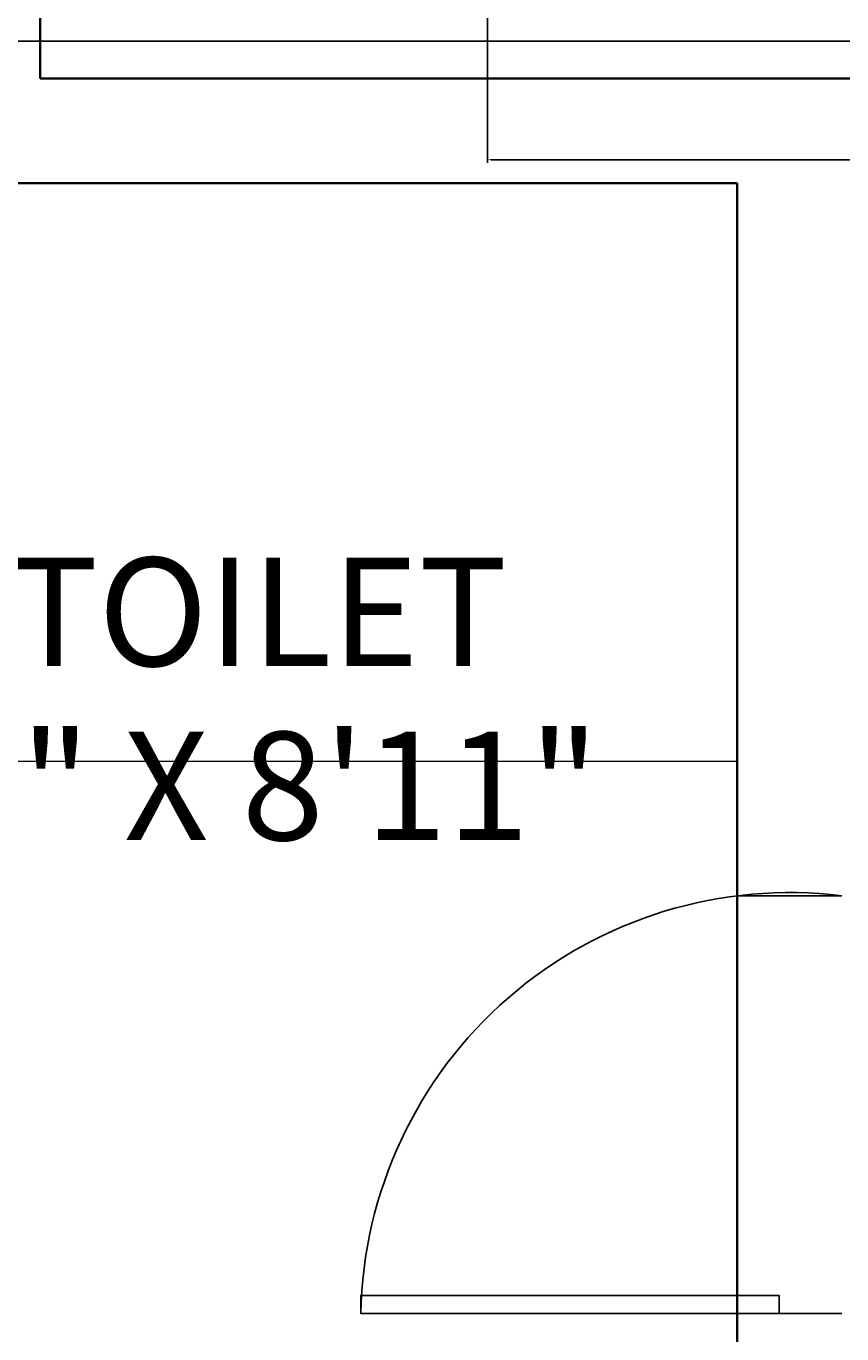
# Model space of a CAD drawing. Units: inches. Extents: x -61 to 1599, y -1316 to 257.
# Tile 62 of 204: x 119 to 166, y -241 to -166. Entities that reach past the tile are written whole.
import ezdxf

# ---------------------------------------------------------------- set-up
doc = ezdxf.new("R2010")
doc.units = ezdxf.units.IN
doc.header["$MEASUREMENT"] = 0
doc.linetypes.add('ACAD_ISO02W100', pattern=[15, 12, -3])
for name, color, linetype, lineweight in [('A-ANNO-DIMS', 2, 'Continuous', 18), ('A-AREA-IDEN', 1, 'Continuous', 18), ('A-FLOR-FIXT', 8, 'Continuous', 18), ('A-WALL-JAMB', 4, 'ACAD_ISO02W100', 25), ('DOORS', 2, 'Continuous', 25), ('WALLS', 4, 'Continuous', 35)]:
    doc.layers.add(name, color=color, linetype=linetype, lineweight=lineweight)
doc.styles.get("Standard").update_dxf_attribs({"font": 'arial.ttf'})
doc.dimstyles.get("Standard").update_dxf_attribs({"dimtxt": 0.18, "dimasz": 0.18, "dimexe": 0.18, "dimexo": 0.0625, "dimgap": 0.09, "dimtad": 0, "dimtih": 1, "dimtoh": 1, "dimdec": 0, "dimzin": 0, "dimdsep": 46, "dimlunit": 3, "dimtxsty": 'Standard', "dimcen": 0.09, "dimadec": 0, "dimazin": 0, "dimtfac": 1, "dimtdec": 0, "dimtofl": 0, "dimtmove": 0, "dimatfit": 3, "dimfxl": 1, "dimtolj": 1, "dimtzin": 0, "dimarcsym": 0})

# ---------------------------------------------------------------- blocks, each defined once
blk = doc.blocks.new('DOOR-SWING-24')
blk.add_line((0, 0), (0, 3.6))
blk.add_lwpolyline([(0, 0), (0, -24), (1.05, -24), (1.05, 0)], close=True)
blk.add_arc((-0.441, 0.618), 24.622, 271.02591, 6.95592)
blk = doc.blocks.new('*D670')
at = {"layer": 'A-ANNO-DIMS', "color": 0, "lineweight": -2, "transparency": 16777216}
for p, q in [((145.375, -161.442), (145.375, -174.159)), ((229.375, -161.442), (229.375, -174.159)), ((145.555, -173.979), (186.47, -173.979)), ((229.195, -173.979), (188.279, -173.979))]:
    blk.add_line(p, q, dxfattribs=at)
at = {"layer": 'A-ANNO-DIMS', "color": 0, "transparency": 16777216}
for points in [[(145.555, -173.949), (145.555, -174.009), (145.375, -173.979)], [(229.195, -173.949), (229.195, -174.009), (229.375, -173.979)]]:
    blk.add_solid(points, dxfattribs=at)
at = {"layer": 'DEFPOINTS', "color": 0, "transparency": 16777216}
for p in [(145.375, -161.379), (229.375, -161.379), (229.375, -173.979)]:
    blk.add_point(p, dxfattribs=at)
at = {"layer": 'A-ANNO-DIMS', "color": 0, "transparency": 16777216, "insert": (187.375, -173.979), "char_height": 0.18, "attachment_point": 5}
blk.add_mtext('\\A1;SOFA 84 TYP.', dxfattribs=at)
blk = doc.blocks.new('*D687')
at = {"layer": 'A-ANNO-DIMS', "color": 0, "lineweight": -2, "transparency": 16777216}
for p, q in [((289.418, 181.677), (-61.077, 181.677)), ((-60.897, 181.497), (-60.897, -528.952)), ((-60.897, -1239.765), (-60.897, -529.316)), ((319.64, -1239.945), (-61.077, -1239.945))]:
    blk.add_line(p, q, dxfattribs=at)
at = {"layer": 'A-ANNO-DIMS', "color": 0, "transparency": 16777216}
for points in [[(-60.927, 181.497), (-60.867, 181.497), (-60.897, 181.677)], [(-60.927, -1239.765), (-60.867, -1239.765), (-60.897, -1239.945)]]:
    blk.add_solid(points, dxfattribs=at)
at = {"layer": 'DEFPOINTS', "color": 0, "transparency": 16777216}
for p in [(289.481, 181.677), (-60.897, -1239.945), (319.703, -1239.945)]:
    blk.add_point(p, dxfattribs=at)
at = {"layer": 'A-ANNO-DIMS', "color": 0, "transparency": 16777216, "insert": (-60.897, -529.134), "char_height": 0.18, "attachment_point": 5}
blk.add_mtext('\\A1;1421.6', dxfattribs=at)
blk = doc.blocks.new('*D699')
at = {"layer": 'A-ANNO-DIMS', "color": 0, "lineweight": -2, "transparency": 16777216}
for p, q in [((835.64, -167.169), (-61.077, -167.169)), ((-60.897, -167.349), (-60.897, -306.726)), ((-60.897, -446.466), (-60.897, -307.09)), ((841.64, -446.646), (-61.077, -446.646))]:
    blk.add_line(p, q, dxfattribs=at)
at = {"layer": 'A-ANNO-DIMS', "color": 0, "transparency": 16777216}
for points in [[(-60.927, -167.349), (-60.867, -167.349), (-60.897, -167.169)], [(-60.927, -446.466), (-60.867, -446.466), (-60.897, -446.646)]]:
    blk.add_solid(points, dxfattribs=at)
at = {"layer": 'DEFPOINTS', "color": 0, "transparency": 16777216}
for p in [(835.703, -167.169), (-60.897, -446.646), (841.703, -446.646)]:
    blk.add_point(p, dxfattribs=at)
at = {"layer": 'A-ANNO-DIMS', "color": 0, "transparency": 16777216, "insert": (-60.897, -306.908), "char_height": 0.18, "attachment_point": 5}
blk.add_mtext('\\A1;279.5', dxfattribs=at)
blk = doc.blocks.new('*D700')
at = {"layer": 'A-ANNO-DIMS', "color": 0, "lineweight": -2, "transparency": 16777216}
for p, q in [((14.703, -616.882), (14.703, 257.457)), ((14.883, 257.277), (96.772, 257.277)), ((179.572, 257.277), (97.683, 257.277)), ((179.752, -616.882), (179.752, 257.457))]:
    blk.add_line(p, q, dxfattribs=at)
at = {"layer": 'A-ANNO-DIMS', "color": 0, "transparency": 16777216}
for points in [[(14.883, 257.307), (14.883, 257.247), (14.703, 257.277)], [(179.572, 257.307), (179.572, 257.247), (179.752, 257.277)]]:
    blk.add_solid(points, dxfattribs=at)
at = {"layer": 'DEFPOINTS', "color": 0, "transparency": 16777216}
for p in [(179.752, 257.277), (14.703, -616.945), (179.752, -616.945)]:
    blk.add_point(p, dxfattribs=at)
at = {"layer": 'A-ANNO-DIMS', "color": 0, "transparency": 16777216, "insert": (97.227, 257.277), "char_height": 0.18, "attachment_point": 5}
blk.add_mtext('\\A1;165.05', dxfattribs=at)

msp = doc.modelspace()

# ---------------------------------------------------------------- linework, layer by layer
at = {"layer": 'A-FLOR-FIXT'}
msp.add_line((87.7028, -208.5091), (159.7028, -208.5091), dxfattribs=at)
at = {"layer": 'A-WALL-JAMB'}
for p, q in [((165.7028, -216.2369), (159.7028, -216.2369)), ((165.7028, -240.2369), (159.7028, -240.2369))]:
    msp.add_line(p, q, dxfattribs=at)
at = {"layer": 'WALLS'}
for p, q in [((119.7028, -169.3229), (119.7028, -13.3229)), ((119.7028, -169.3229), (234.7028, -169.3229)), ((87.7028, -175.3229), (159.7028, -175.3229)), ((159.7028, -282.3229), (159.7028, -175.3229))]:
    msp.add_line(p, q, dxfattribs=at)

# ---------------------------------------------------------------- block references
at = {"layer": 'DOORS', "extrusion": (0, 0, -1), "zscale": -1, "rotation": 89.99999999999957}
msp.add_blockref('DOOR-SWING-24', (-162.1028, -240.2369), dxfattribs=at)

# ---------------------------------------------------------------- texts
at = {"layer": 'A-AREA-IDEN'}
for s, p in [(' M . TOILET', (102.978, -203.0507)), ('  6\'0" X 8\'11"', (102.978, -213.0484))]:
    msp.add_text(s, height=6.223643, dxfattribs=at).set_placement(p)

# ---------------------------------------------------------------- dimensions: what is measured, and where the dimension line sits
at = {"layer": 'A-ANNO-DIMS'}
dim = msp.add_linear_dim(base=(179.7521, 257.2771), p1=(14.7028, -616.9446), p2=(179.7521, -616.9446), dimstyle='Standard', override={"dimdec": 2, "dimlfac": 1, "dimrnd": 0, "dimzin": 0, "dimdsep": 46, "dimlunit": 2}, dxfattribs=at)
dim.commit()
dim.dimension.update_dxf_attribs({"geometry": '*D700', "text_midpoint": (97.2274, 257.2771)})
for base, p1, p2, picture, middle in [((-60.8972, -1239.9446), (289.4807, 181.6771), (319.7028, -1239.9446), '*D687', (-60.8972, -529.1337)), ((-60.8972, -446.6462), (835.7028, -167.169), (841.7028, -446.6462), '*D699', (-60.8972, -306.9076))]:
    dim = msp.add_linear_dim(base=base, p1=p1, p2=p2, angle=90, dimstyle='Standard', override={"dimdec": 1, "dimlfac": 1, "dimrnd": 0, "dimzin": 0, "dimdsep": 46, "dimlunit": 2}, dxfattribs=at)
    dim.commit()
    dim.dimension.update_dxf_attribs({"geometry": picture, "text_midpoint": middle})
dim = msp.add_linear_dim(base=(229.3746, -173.9792), p1=(145.3746, -161.3792), p2=(229.3746, -161.3792), text='SOFA <> TYP.', dimstyle='Standard', override={"dimdec": 0, "dimlfac": 1, "dimrnd": 0, "dimzin": 0, "dimdsep": 46, "dimlunit": 2}, dxfattribs=at)
dim.commit()
dim.dimension.update_dxf_attribs({"geometry": '*D670', "text_midpoint": (187.3746, -173.9792)})

doc.saveas('drawing.dxf')
